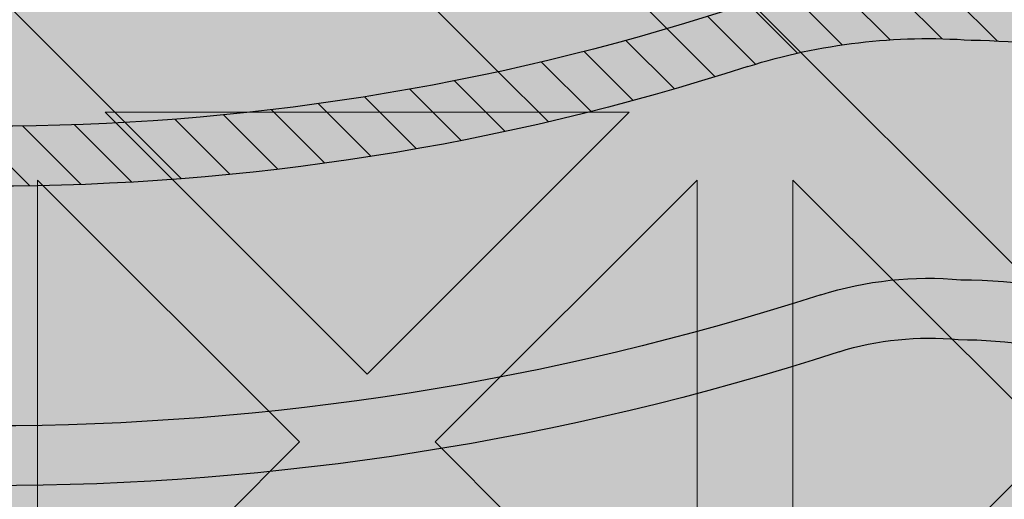
# Model space of a CAD drawing. Units: inches. Extents: x 844 to 2234, y 346 to 1084.
# Tile 28 of 93: x 1257.455 to 1260.074, y 687.38 to 688.657. Entities that reach past the tile are written whole.
import ezdxf

# ---------------------------------------------------------------- set-up
doc = ezdxf.new("R2010")
doc.units = ezdxf.units.IN
doc.header["$MEASUREMENT"] = 0
doc.layers.add('furniture', color=8, linetype='Continuous', lineweight=18)
doc.layers.add('RA-AP-01$0$INT', color=35, linetype='Continuous', lineweight=5)
doc.layers.add('RA-AP-01$0$FURN', color=3, linetype='Continuous')
doc.layers.add('RA-AP-01$0$WOOD', color=64, linetype='Continuous')

# ---------------------------------------------------------------- blocks, each defined once
blk = doc.blocks.new('A$C18D01794')
at = {"layer": 'RA-AP-01$0$INT'}
h = blk.add_hatch(color=256, dxfattribs=at)
h.paths.add_polyline_path([(4.585917135068449, -6.356712009588271), (4.555206456959269, -6.35671200958746), (4.555206456959137, -6.387422687716308), (4.874495778835233, -6.706712009592356), (4.90520645695423, -6.676001331474049)])
h.paths.add_polyline_path([(5.255206456948813, -6.387422687716306), (5.255206456948682, -6.356712009605972), (5.224495778822613, -6.356712009605161), (4.905206456953498, -6.676001331474273), (4.935917135072151, -6.706712009592924)])
h.paths.add_polyline_path([(4.935917135072559, -6.706712009592068), (4.905206456953564, -6.737422687710376), (5.255206456951813, -7.087422687708613), (5.255206456951549, -7.026001331471008)])
h.paths.add_polyline_path([(4.555206456956399, -7.026001331471013), (4.555206456956134, -7.087422687708616), (4.905206456953821, -6.737422687710943), (4.874495778835166, -6.70671200959229)])
h = blk.add_hatch(color=256, dxfattribs=at)
h.paths.add_polyline_path([(4.585917135068448, -6.356712009588273), (4.614201406330596, -6.356712009589021), (4.668846067270487, -6.411356670531338), (4.723490728212344, -6.356712009591912), (4.771774999457151, -6.35671200959319), (4.826419660396886, -6.411356670535356), (4.862780050090322, -6.374996280843536), (4.844495778842715, -6.356712009595112), (4.862780050090411, -6.356712009595595), (4.905206456960182, -6.399138416468211), (4.947632863832445, -6.356712009597838), (4.965917135079675, -6.356712009598322), (4.947632863831759, -6.374996280845421), (4.983993253523576, -6.411356670538857), (5.038637914464627, -6.356712009600247), (5.08692218571208, -6.356712009601523), (5.141566846649976, -6.411356670541852), (5.196211507589851, -6.356712009604411), (5.224495778822615, -6.356712009605161), (4.905206456953975, -6.676001331473793)])
h.paths.add_polyline_path([(4.895206456956031, -6.637717060225675), (4.895206456958921, -6.528427738347902), (4.840561796018589, -6.583072399285802)], flags=16)
h.paths.add_polyline_path([(4.915206456955638, -6.637717060226121), (4.969851117895509, -6.583072399288678), (4.915206456957609, -6.528427738348344)], flags=16)
h.paths.add_polyline_path([(4.826419660395175, -6.568930263661755), (4.881064321335613, -6.514285602723745), (4.771774999456703, -6.514285602720857)], flags=16)
h.paths.add_polyline_path([(4.983993253519558, -6.568930263665262), (5.038637914460456, -6.514285602726792), (4.929348592581548, -6.514285602724816)], flags=16)
h.paths.add_polyline_path([(4.881064321336025, -6.494285602723742), (4.826419660397532, -6.439640941782821), (4.771774999457062, -6.494285602720859)], flags=16)
h.paths.add_polyline_path([(4.929348592582019, -6.494285602724817), (5.038637914460982, -6.494285602726792), (4.983993253522945, -6.439640941786327)], flags=16)
h.paths.add_polyline_path([(4.895206456960191, -6.480143467100443), (4.895206456962115, -6.407422687715913), (4.876922185715016, -6.389138416467584), (4.840561796021581, -6.425498806159401)], flags=16)
h.paths.add_polyline_path([(4.915206456958487, -6.480143467100889), (4.969851117899527, -6.425498806162279), (4.933490728206909, -6.389138416468043), (4.9152064569598, -6.40742268771434)], flags=16)
h.paths.add_polyline_path([(4.757632863832376, -6.480143467096812), (4.812277524772842, -6.425498806158772), (4.757632863834348, -6.370854145217844)], flags=16)
h.paths.add_polyline_path([(4.737632863832376, -6.480143467096286), (4.737632863834348, -6.370854145217375), (4.682988202893906, -6.425498806155385)], flags=16)
h.paths.add_polyline_path([(5.05278005008503, -6.480143467103376), (5.052780050087917, -6.370854145224413), (4.998135389146995, -6.425498806162908)], flags=16)
h.paths.add_polyline_path([(5.072780050085024, -6.480143467103744), (5.127424711025931, -6.42549880616527), (5.072780050087916, -6.370854145224832)], flags=16)
h.paths.add_polyline_path([(4.935917135072783, -6.706712009592292), (5.255206456948811, -6.387422687716309), (5.255206456948932, -6.415706958964177), (5.200561796010279, -6.470351619902839), (5.255206456949403, -6.524996280841948), (5.25520645694961, -6.5732805520894), (5.200561796009787, -6.627925213029239), (5.236922185702417, -6.664285602721864), (5.255206456949919, -6.646001331474357), (5.255206456949998, -6.664285602721898), (5.212780050078687, -6.706712009592262), (5.25520645695036, -6.749138416463932), (5.255206456950438, -6.767422687711313), (5.236922185702424, -6.749138416463297), (5.200561796009796, -6.785498806155928), (5.255206456950753, -6.840143467096874), (5.25520645695096, -6.888427738341682), (5.200561796010322, -6.943072399282328), (5.255206456951428, -6.997717060223427), (5.255206456951547, -7.026001331471006)])
h.paths.add_polyline_path([(5.042988202883395, -6.785498806155427), (5.097632863823085, -6.840143467095101), (5.097632863822622, -6.730854145216193)], flags=16)
h.paths.add_polyline_path([(5.028846067259663, -6.771356670531693), (5.083490728198774, -6.716712009592573), (4.974201406321001, -6.716712009593042)], flags=16)
h.paths.add_polyline_path([(5.117632863823087, -6.840143467095186), (5.172277524762331, -6.785498806155926), (5.11763286382262, -6.730854145216225)], flags=16)
h.paths.add_polyline_path([(5.08349072819877, -6.696712009593886), (5.028846067259652, -6.642067348654775), (4.974201406320998, -6.696712009593438)], flags=16)
h.paths.add_polyline_path([(5.131774999446817, -6.854285602718917), (5.186419660386065, -6.799640941779662), (5.241064321325782, -6.854285602719365)], flags=17)
h.paths.add_polyline_path([(5.131774999446228, -6.716712009592374), (5.186419660386065, -6.771356670532194), (5.222780050079488, -6.734996280838764), (5.204495778832781, -6.716712009592063)], flags=16)
h.paths.add_polyline_path([(5.097632863822613, -6.682569873970264), (5.097632863823061, -6.573280552091354), (5.042988202883383, -6.627925213031044)], flags=16)
h.paths.add_polyline_path([(5.131774999446899, -6.874285602718915), (5.241064321325809, -6.874285602719364), (5.186419660386591, -6.928930263658598)], flags=17)
h.paths.add_polyline_path([(5.131774999446226, -6.696712009594078), (5.204495778830767, -6.696712009594374), (5.22278005007868, -6.67842773834687), (5.186419660386049, -6.642067348654249)], flags=16)
h.paths.add_polyline_path([(5.11763286382262, -6.682569873970225), (5.17227752476232, -6.627925213030515), (5.117632863823064, -6.573280552091267)], flags=16)
h.paths.add_polyline_path([(5.186419660386069, -6.613783077405491), (5.241064321325754, -6.559138416465795), (5.131774999446791, -6.559138416466263)], flags=16)
h.paths.add_polyline_path([(5.131774999446872, -6.539138416466263), (5.24106432132578, -6.539138416465794), (5.186419660386554, -6.484493755526573)], flags=16)
h.paths.add_polyline_path([(5.255206456951811, -7.08742268770861), (5.255206456951895, -7.106712009588038), (4.555206456956052, -7.106712009588038), (4.555206456956136, -7.087422687708617), (4.905206456953973, -6.737422687710788)])
h.paths.add_polyline_path([(4.983993253513404, -6.8444937555241), (4.92934859257295, -6.899138416462108), (5.03863791445186, -6.899138416465014)], flags=16)
h.paths.add_polyline_path([(4.969851117889988, -6.83035161990006), (4.915206456952556, -6.775706958960171), (4.915206456949648, -6.884996280837944)], flags=16)
h.paths.add_polyline_path([(4.929348592572535, -6.919138416462105), (4.983993253511019, -6.973783077403037), (5.038637914451496, -6.919138416465012)], flags=16)
h.paths.add_polyline_path([(5.052780050074912, -6.93328055208906), (4.998135389134438, -6.987925213027088), (5.052780050072919, -7.042569873968025)], flags=16)
h.paths.add_polyline_path([(5.07278005007491, -6.933280552089588), (5.072780050072918, -7.042569873968497), (5.127424711013374, -6.987925213030498)], flags=16)
h.paths.add_polyline_path([(4.89520645695295, -6.775706958959721), (4.840561796013067, -6.830351619897157), (4.895206456950961, -6.884996280837494)], flags=16)
h.paths.add_polyline_path([(4.915206456948365, -6.933280552085403), (4.915206456946434, -7.006001331471951), (4.933490728192729, -7.024285602719066), (4.969851117886972, -6.987925213026453)], flags=16)
h.paths.add_polyline_path([(4.881064321327021, -6.899138416461022), (4.82641966038902, -6.84449375552057), (4.771774999448108, -6.899138416459029)], flags=16)
h.paths.add_polyline_path([(4.895206456950073, -6.933280552084951), (4.840561796009022, -6.987925213023558), (4.876922185700835, -7.024285602716997), (4.895206456948749, -7.006001331469487)], flags=16)
h.paths.add_polyline_path([(4.983993253510392, -7.0020673486505), (4.947632863816944, -7.038427738342319), (4.965917135064043, -7.05671200959023), (5.038637914448995, -7.056712009591555)], flags=16)
h.paths.add_polyline_path([(4.881064321326543, -6.91913841646102), (4.771774999447578, -6.919138416459031), (4.826419660385607, -6.973783077399508)], flags=16)
h.paths.add_polyline_path([(4.905206456946447, -7.014285602717636), (4.862780050074785, -7.056712009588352), (4.947632863816685, -7.056712009589775)], flags=16)
h.paths.add_polyline_path([(5.14156684663679, -7.002067348654549), (5.086922185696452, -7.056712009592438), (5.196211507574223, -7.056712009594425)], flags=16)
h.paths.add_polyline_path([(4.8264196603837, -7.002067348646972), (4.771774999442643, -7.056712009585575), (4.8444957788276, -7.056712009587508), (4.862780050075511, -7.038427738340416)], flags=16)
h.paths.add_polyline_path([(4.812277524760289, -6.98792521302292), (4.757632863822258, -6.933280552082447), (4.757632863819352, -7.042569873961408)], flags=16)
h.paths.add_polyline_path([(4.73763286382226, -6.933280552082079), (4.682988202881349, -6.987925213020536), (4.737632863819352, -7.04256987396099)], flags=16)
h.paths.add_polyline_path([(4.723490728195188, -7.056712009584289), (4.668846067257299, -7.002067348643949), (4.614201406317417, -7.056712009581383)], flags=16)
h.paths.add_polyline_path([(4.597632863829262, -6.706712009592262), (4.555206456957951, -6.664285602721896), (4.555206456958029, -6.646001331474357), (4.573490728205535, -6.664285602721864), (4.609851117898167, -6.627925213029238), (4.555206456958338, -6.573280552089402), (4.555206456958546, -6.524996280841952), (4.60985111789767, -6.470351619902839), (4.555206456959015, -6.415706958964177), (4.555206456959138, -6.387422687716309), (4.874495778835167, -6.70671200959229), (4.5552064569564, -7.026001331471015), (4.555206456956523, -6.997717060223433), (4.609851117897629, -6.94307239928233), (4.555206456956988, -6.888427738341681), (4.555206456957198, -6.840143467096881), (4.609851117898153, -6.78549880615593), (4.573490728205528, -6.749138416463297), (4.555206456957507, -6.76742268771132), (4.555206456957585, -6.749138416463933)])
h.paths.add_polyline_path([(4.712780050085332, -6.730854145216195), (4.712780050084863, -6.840143467095105), (4.767424711024555, -6.785498806155427)], flags=16)
h.paths.add_polyline_path([(4.726922185709173, -6.716712009592573), (4.781566846648288, -6.771356670531693), (4.836211507586949, -6.716712009593043)], flags=16)
h.paths.add_polyline_path([(4.692780050085327, -6.730854145216225), (4.638135389145619, -6.785498806155928), (4.692780050084865, -6.840143467095185)], flags=16)
h.paths.add_polyline_path([(4.726922185709182, -6.696712009593886), (4.836211507586949, -6.696712009593436), (4.7815668466483, -6.642067348654773)], flags=16)
h.paths.add_polyline_path([(4.678637914461726, -6.71671200959237), (4.605917135075169, -6.716712009592063), (4.587632863828464, -6.734996280838766), (4.623993253521887, -6.771356670532195)], flags=16)
h.paths.add_polyline_path([(4.712780050085336, -6.68256987397026), (4.767424711024568, -6.627925213031042), (4.71278005008489, -6.573280552091352)], flags=16)
h.paths.add_polyline_path([(4.678637914461726, -6.696712009594076), (4.623993253521899, -6.642067348654247), (4.587632863829271, -6.67842773834687), (4.605917135077185, -6.696712009594376)], flags=16)
h.paths.add_polyline_path([(4.692780050085336, -6.682569873970228), (4.692780050084889, -6.573280552091267), (4.638135389145632, -6.627925213030515)], flags=16)
h.paths.add_polyline_path([(4.623993253521885, -6.799640941779662), (4.678637914461131, -6.854285602718915), (4.56934859258217, -6.854285602719365)], flags=17)
h.paths.add_polyline_path([(4.623993253521901, -6.613783077405509), (4.678637914461158, -6.559138416466263), (4.569348592582195, -6.559138416465795)], flags=16)
h.paths.add_polyline_path([(4.678637914461051, -6.874285602718915), (4.623993253521361, -6.928930263658598), (4.569348592582143, -6.874285602719364)], flags=17)
h.paths.add_polyline_path([(4.678637914461076, -6.539138416466263), (4.623993253521399, -6.484493755526573), (4.569348592582167, -6.539138416465796)], flags=16)
h = blk.add_hatch(color=256, dxfattribs=at)
h.paths.add_polyline_path([(4.969851117891331, -6.583072399286455), (4.915206456952669, -6.63771706022511), (4.915206456952222, -6.528427738347337)])
h.paths.add_polyline_path([(4.895206456953064, -6.637717060225108), (4.840561796014413, -6.583072399286448), (4.895206456953533, -6.528427738347335)])
h.paths.add_polyline_path([(4.826419660390684, -6.568930263662714), (4.771774999451003, -6.514285602723024), (4.881064321329913, -6.514285602723489)])
h.paths.add_polyline_path([(4.881064321329884, -6.494285602723492), (4.771774999450921, -6.494285602723024), (4.82641966039018, -6.439640941783778)])
h.paths.add_polyline_path([(4.895206456953734, -6.48014346709988), (4.840561796013912, -6.425498806160046), (4.876922185707337, -6.389138416466622), (4.895206456954043, -6.40742268771333)])
h.paths.add_polyline_path([(4.862780050082808, -6.374996280843689), (4.826419660390178, -6.411356670536314), (4.771774999450351, -6.356712009596481), (4.844495778835303, -6.356712009596181)])
h.paths.add_polyline_path([(4.812277524766446, -6.425498806160041), (4.757632863827191, -6.480143467099289), (4.757632863826741, -6.370854145220329)])
h.paths.add_polyline_path([(4.737632863827191, -6.480143467099214), (4.682988202887508, -6.425498806159518), (4.737632863826743, -6.370854145220299)])
h.paths.add_polyline_path([(4.668846067263777, -6.41135667053579), (4.614201406325123, -6.356712009597128), (4.723490728202894, -6.356712009596675)])
h.paths.add_polyline_path([(4.905206456953846, -6.399138416467422), (4.862780050082654, -6.356712009596229), (4.947632863824561, -6.356712009595756)])
h.paths.add_polyline_path([(4.915206456952028, -6.480143467099882), (4.91520645695173, -6.407422687715346), (4.933490728199234, -6.389138416467428), (4.96985111789186, -6.425498806160055)])
h.paths.add_polyline_path([(5.038637914454841, -6.494285602723048), (4.929348592575874, -6.494285602723497), (4.983993253515593, -6.439640941783787)])
h.paths.add_polyline_path([(4.983993253515065, -6.568930263662725), (4.929348592575849, -6.514285602723495), (5.038637914454755, -6.514285602723045)])
h.paths.add_polyline_path([(5.052780050079843, -6.480143467099317), (4.998135389140595, -6.425498806160058), (5.052780050080309, -6.370854145220356)])
h.paths.add_polyline_path([(4.983993253516868, -6.411356670536324), (4.947632863824241, -6.374996280843694), (4.965917135071747, -6.356712009596188), (5.038637914456701, -6.356712009596504)])
h.paths.add_polyline_path([(5.127424711019533, -6.425498806159557), (5.072780050079843, -6.480143467099239), (5.07278005008031, -6.370854145220326)])
h.paths.add_polyline_path([(5.141566846643269, -6.411356670535829), (5.086922185704154, -6.356712009596707), (5.196211507581929, -6.356712009597176)])
for p, q in [((4.905206456953975, -6.676001331473793), (4.585917135071132, -6.356712009590955)), ((4.737632863834348, -6.370854145217375), (4.682988202893906, -6.425498806155385)), ((4.737632863832376, -6.480143467096285), (4.737632863834348, -6.370854145217375)), ((4.757632863832376, -6.48014346709681), (4.757632863834348, -6.370854145217847)), ((4.757632863834348, -6.370854145217847), (4.812277524772842, -6.425498806158774)), ((4.840561796021581, -6.425498806159403), (4.876922185715016, -6.389138416467584)), ((4.895206456962113, -6.407422687715495), (4.895206456960191, -6.480143467100447)), ((4.682988202893908, -6.425498806155387), (4.737632863832376, -6.480143467096285)), ((4.757632863832376, -6.48014346709681), (4.812277524772842, -6.425498806158774)), ((4.895206456960191, -6.480143467100447), (4.840561796021581, -6.425498806159401)), ((4.771774999457064, -6.494285602720857), (4.826419660397532, -6.439640941782821)), ((4.881064321336027, -6.494285602723744), (4.826419660397532, -6.439640941782821)), ((4.771774999457064, -6.494285602720857), (4.881064321336027, -6.494285602723744))]:
    blk.add_line(p, q, dxfattribs=at)
blk = doc.blocks.new('A$C32926AE1')
at = {"layer": 'RA-AP-01$0$WOOD'}
h = blk.add_hatch(color=256, dxfattribs=at)
h.dxf.hatch_style = 1
h.paths.add_polyline_path([(5.157430609644524, 4.573483066760929, -0.1009492694046607), (5.155401577623758, 4.593365984175333, -0.1842662638101597), (5.172249623284174, 4.638795604568598, 0.2056608120311276), (5.179560981299304, 4.661316324430096, 0.3614336704623542), (5.134352340494423, 4.706524965234944, 0.2056608120311297), (5.111831620632933, 4.699213607219793, -0.1842662638101113), (5.066402000239693, 4.682365561559342, -0.1055311479399994), (5.045656153913092, 4.68467289944697, 0.1567636581983829), (4.763886414745334, 4.684672899446966, -0.1055311479399895), (4.743140568418733, 4.68236556155934, -0.1842662638100833), (4.6977109480255, 4.69921360721979, 0.2056608120302612), (4.675190228164109, 4.706524965234949, 0.3614336704708441), (4.629981587358889, 4.66131632442871, 0.2056608120245944), (4.637292945374126, 4.638795604567974, -0.1842662638101024), (4.654140991034615, 4.59336598417475, -0.1009492694055169), (4.652111959013835, 4.573483066760181, 0.021410119221476), (4.629748025606143, 4.156712009541676, 0.0214101192214795), (4.652111959013809, 3.739940952323101, -0.1009492694059586), (4.654140991034615, 3.720058034908448, -0.1842662638100975), (4.637292945374126, 3.674628414515226, 0.2056608120245705), (4.629981587358889, 3.652107694654492, 0.3614336704708879), (4.675190228164113, 3.606899053848249, 0.2056608120302384), (4.697710948025501, 3.614210411863408, -0.1842662638100995), (4.743140568418738, 3.63105845752386, -0.1055311479402541), (4.763886414745388, 3.628751119636215, 0.1567636581983776), (5.045656153913137, 3.628751119636244, -0.1055311479397538), (5.066402000239692, 3.631058457523857, -0.1842662638101067), (5.111831620632931, 3.614210411863407, 0.2056608120310924), (5.134352340494417, 3.606899053848256, 0.3614336704624001), (5.179560981299307, 3.652107694653103, 0.2056608120311314), (5.172249623284175, 3.6746284145146, -0.1842662638101402), (5.155401577623758, 3.72005803490786, -0.1009492694051366), (5.15743060964455, 3.739940952322354, 0.0214101192215073), (5.179794543052287, 4.156712009541468, 0.0214101192215252)])
h.paths.add_polyline_path([(4.639748609479751, 4.156712009541513, 0.0213537860821624), (4.661970494867118, 3.741887061152232, -0.094075836301374), (4.664143710413708, 3.7196126951003, -0.1824818158568985), (4.644813765429836, 3.668037719127816, 0.2056608120245319), (4.639939526753007, 3.653023905887301, 0.3614336704710246), (4.676106439397173, 3.616856993242342, 0.2056608120302234), (4.691120252638095, 3.621731231919122, -0.1824818158602558), (4.742695228611606, 3.641061176902986, -0.1029891339458722), (4.766991894714349, 3.638256818950944, 0.156709409989566), (5.042550673941472, 3.638256818950105, -0.102989133958497), (5.066847340047078, 3.641061176902949, -0.1824818158594995), (5.118422316020358, 3.621731231919103, 0.2056608120311416), (5.133436129261316, 3.616856993242346, 0.3614336704621468), (5.169603041905217, 3.653023905886178, 0.2056608120310986), (5.164728803228477, 3.668037719127177, -0.1824818158565612), (5.145398858244737, 3.719612695099578, -0.0940758363009313), (5.147572073791232, 3.741887061151398, 0.0213537860822023), (5.169793959178681, 4.156712009541451, 0.0213537860822226), (5.147572073791203, 4.571536957931898, -0.0940758363005034), (5.145398858244737, 4.59381132398362, -0.1824818158565587), (5.164728803228476, 4.645386299956021, 0.2056608120311045), (5.169603041905216, 4.66040011319702, 0.3614336704621845), (5.133436129261313, 4.696567025840856, 0.2056608120310773), (5.118422316020359, 4.691692787164098, -0.182481815859508), (5.066847340047078, 4.67236284218025, -0.1029891339584606), (5.04255067394148, 4.675167200133092, 0.156709409989566), (4.766991894714357, 4.675167200132257, -0.1029891339458842), (4.742695228611611, 4.672362842180213, -0.1824818158602725), (4.691120252638095, 4.691692787164077, 0.2056608120302152), (4.676106439397174, 4.696567025840858, 0.3614336704710363), (4.639939526753005, 4.660400113195899, 0.2056608120245495), (4.644813765429837, 4.645386299955384, -0.1824818158568934), (4.664143710413708, 4.593811323982902, -0.0940758363009187), (4.661970494867149, 4.571536957931074, 0.021353786082177)], flags=16)
h.paths.add_polyline_path([(5.129794543052235, 4.432167055276933, -0.0141661062790638), (5.130152669293814, 4.156927903047693, -0.0141661062790647), (5.129794543052234, 3.881688750818433, -0.0785247771143638), (5.10979738006795, 3.755143611847103, 0.0945969212073497), (5.105408519571111, 3.717898134952927, 0.1043170707844957), (5.116074640131521, 3.670385395016088, 0.1043170707864965), (5.068561900193738, 3.681051515576561, 0.09459692119553), (5.031316423304057, 3.676662655080835, -0.1580239521427272), (4.778226145355827, 3.676662655080367, 0.0945969211986668), (4.740980668464973, 3.681051515576592, 0.1043170707882822), (4.693467928526415, 3.670385395015844, 0.1043170707867916), (4.704134049087309, 3.717898134953662, 0.0945969211972894), (4.69974518859162, 3.755143611844042, -0.0785247771163196), (4.679748025606343, 3.881688750818406, -0.0141661062790663), (4.679389899364763, 4.156927903047693, -0.0141661062790672), (4.679748025606343, 4.432167055276998, -0.0785247771163064), (4.699745188591625, 4.55871219425134, 0.094596921197333), (4.704134049087308, 4.595957671141738, 0.1043170707867205), (4.693467928526416, 4.643470411079523, 0.1043170707882628), (4.740980668464965, 4.632804290518776, 0.0945969211988114), (4.778226145355874, 4.637193151015016, -0.158023952142669), (5.031316423304015, 4.637193151014546, 0.0945969211956361), (5.068561900193736, 4.632804290518806, 0.1043170707864979), (5.11607464013152, 4.643470411079278, 0.1043170707844617), (5.105408519571112, 4.595957671142455, 0.0945969212074597), (5.109797380067959, 4.558712194248236, -0.0785247771143467)], flags=0)
h.paths.add_polyline_path([(5.119794532311105, 4.432259799204851, -0.0142000800617244), (5.120156169157484, 4.156927903047701, -0.0142000800617277), (5.119794532311105, 3.881596006890482, -0.0784894509520253), (5.100273383573699, 3.758192358677797, 0.0940138827242913), (5.095413455884425, 3.717477693979438, 0.0606271852308753), (5.099615656341024, 3.686844378806616, 0.0606271852322524), (5.068982341167493, 3.691046579263239, 0.0940138827010453), (5.028267676478798, 3.686186651576848, -0.1580706864508061), (4.781274892180912, 3.686186651576435, 0.0940138827026903), (4.740560227491556, 3.691046579263279, 0.0606271852339895), (4.709926912317155, 3.686844378806508, 0.0606271852329405), (4.714129112773991, 3.717477693980356, 0.094013882701304), (4.709269185087677, 3.758192358669163, -0.0784894509577193), (4.689748036347473, 3.881596006890469, -0.014200080061729), (4.689386399501094, 4.156927903047709, -0.0142000800617217), (4.689748036347473, 4.432259799204808, -0.078489450957724), (4.709269185087651, 4.555663447426125, 0.0940138827014585), (4.714129112773992, 4.596378112114996, 0.0606271852329731), (4.709926912317154, 4.62701142728886, 0.0606271852340196), (4.74056022749157, 4.622809226832087, 0.0940138827024997), (4.781274892180847, 4.627669154518912, -0.1580706864508359), (5.028267676478777, 4.627669154518526, 0.0940138827010946), (5.068982341167492, 4.622809226832129, 0.060627185232254), (5.099615656341024, 4.627011427288751, 0.0606271852308727), (5.095413455884425, 4.59637811211593, 0.0940138827241088), (5.100273383573675, 4.555663447417647, -0.0784894509520978)], flags=0)
h.paths.add_polyline_path([(5.06978912287499, 4.430218106756144, -0.014241683694547), (5.070173729147532, 4.156927903047672, -0.0142416836945458), (5.06978912287499, 3.883637699339223, -0.0800609523125196), (5.052662118612511, 3.773463122773442, 0.0526421978001116), (5.04590916754064, 3.740550867606997, 0.0526421977992423), (5.012996912374707, 3.73379791653534, -0.1583028414718258), (4.796545656286308, 3.73379791653451, 0.0526421978034211), (4.763633401117837, 3.740550867607021, 0.0526421978018622), (4.756880450045755, 3.773463122774558, -0.0800609523117106), (4.739753445783639, 3.883637699339268, -0.0142416836945435), (4.739368839511098, 4.156927903047671, -0.0142416836945477), (4.739753445783639, 4.430218106756155, -0.0800609523116345), (4.75688045004574, 4.540392683320762, 0.052642197801941), (4.763633401117837, 4.573304938488346, 0.0526421978035071), (4.796545656286361, 4.580057889560873, -0.1583028414717561), (5.012996912374669, 4.580057889560039, 0.0526421977993048), (5.04590916754064, 4.57330493848837, 0.0526421978002057), (5.052662118612529, 4.540392683321868, -0.080060952312477)], flags=0)
h.paths.add_polyline_path([(5.049789715110557, 4.43038092723357, -0.0143097550741839), (5.05018085590259, 4.156927903047715, -0.0143097550741854), (5.049789715110558, 3.883474878861827, -0.0800685599149176), (5.03362098255317, 3.779581877367999, 0.0306258898956367), (5.028241146483733, 3.758218888663947, 0.0306258898977031), (5.006878157778253, 3.75283905259408, -0.1583983521624096), (4.802664410878162, 3.752839052594731, 0.0306258898946014), (4.781301422174808, 3.758218888663924, 0.0306258898967912), (4.775921586105202, 3.779581877368794, -0.080068559914251), (4.759752853548071, 3.883474878861786, -0.0143097550741854), (4.759361712756037, 4.156927903047671, -0.0143097550741854), (4.759752853548071, 4.430380927233557, -0.0800685599142479), (4.775921586105193, 4.534273928726546, 0.0306258898968306), (4.781301422174808, 4.555636917431444, 0.0306258898945754), (4.802664410878143, 4.561016753500631, -0.1583983521624168), (5.006878157778244, 4.561016753501291, 0.0306258898977177), (5.028241146483733, 4.555636917431421, 0.0306258898958182), (5.03362098255321, 4.534273928727244, -0.080068559914796)], flags=0)
h.paths.add_polyline_path([(4.999766070382627, 4.428171244713864, -0.0143443147609634), (5.000198441819402, 4.156927903047689, -0.0143443147609612), (4.999766070382627, 3.885684561381556, -0.0784641635803329), (4.987356730658798, 3.799103304488872, -0.1506053783831347), (4.822185837999821, 3.79910330448882, -0.0784641635803318), (4.809776498276007, 3.885684561381509, -0.014344314760963), (4.809344126839227, 4.156927903047677, -0.0143443147609645), (4.809776498276007, 4.428171244713873, -0.0784641635803192), (4.822185837999822, 4.514752501606549, -0.1506053783831338), (4.987356730658798, 4.514752501606494, -0.078464163580285)], flags=0)
h.paths.add_polyline_path([(4.979755254238824, 4.42764379880488, -0.0143772539198268), (4.980205517789977, 4.156927903047693, -0.0143772539198275), (4.979755254238824, 3.886212007290489, -0.0689242507424422), (4.971183264704897, 3.815276770442801, -0.1296645318904179), (4.838359303953726, 3.815276770442746, -0.0689242507424186), (4.829787314419809, 3.886212007290419, -0.0143772539198292), (4.829337050868653, 4.156927903047653, -0.0143772539198325), (4.829787314419809, 4.427643798804946, -0.0689242507424211), (4.838359303953725, 4.498579035652621, -0.1296645318904187), (4.971183264704897, 4.498579035652565, -0.0689242507424401)], flags=0)
h = blk.add_hatch(color=256, dxfattribs=at)
h.dxf.hatch_style = 1
h.paths.add_polyline_path([(5.145398858244737, 4.59381132398362, -0.1824818158565616), (5.164728803228476, 4.645386299956021, 0.2056608120311045), (5.169603041905216, 4.66040011319702, 0.3614336704621845), (5.133436129261313, 4.696567025840856, 0.2056608120310773), (5.118422316020359, 4.691692787164098, -0.182481815859508), (5.066847340047078, 4.67236284218025, -0.1029891339584606), (5.04255067394148, 4.675167200133092, 0.156709409989566), (4.766991894714357, 4.675167200132257, -0.1029891339458842), (4.742695228611611, 4.672362842180213, -0.1824818158602725), (4.691120252638095, 4.691692787164077, 0.2056608120302152), (4.676106439397174, 4.696567025840858, 0.3614336704710363), (4.639939526753005, 4.660400113195899, 0.2056608120245495), (4.644813765429837, 4.645386299955384, -0.1824818158568934), (4.664143710413708, 4.593811323982902, -0.0940758363009187), (4.661970494867149, 4.571536957931074, 0.0213537860821772), (4.639748609479751, 4.156712009541507, 0.0213537860821625), (4.661970494867119, 3.741887061152226, -0.0940758363013071), (4.664143710413708, 3.719612695100309, -0.1824818158569294), (4.644813765429836, 3.668037719127816, 0.2056608120245319), (4.639939526753007, 3.653023905887301, 0.3614336704710246), (4.676106439397173, 3.616856993242342, 0.2056608120302234), (4.691120252638095, 3.621731231919122, -0.1824818158602558), (4.742695228611606, 3.641061176902986, -0.1029891339458722), (4.766991894714349, 3.638256818950944, 0.156709409989566), (5.042550673941472, 3.638256818950105, -0.102989133958497), (5.066847340047078, 3.641061176902949, -0.1824818158594995), (5.118422316020358, 3.621731231919103, 0.2056608120311416), (5.133436129261316, 3.616856993242346, 0.3614336704621468), (5.169603041905217, 3.653023905886178, 0.2056608120310986), (5.164728803228477, 3.668037719127177, -0.1824818158565612), (5.145398858244737, 3.719612695099578, -0.0940758363009313), (5.147572073791232, 3.741887061151398, 0.0213537860822023), (5.169793959178681, 4.156712009541451, 0.0213537860822226), (5.147572073791203, 4.571536957931898, -0.0940758363004996)])
h.paths.add_polyline_path([(5.109797380067958, 4.55871219424824, -0.0785247771143472), (5.129794543052234, 4.432167055276936, -0.0141661062790644), (5.130152669293814, 4.156927903047685, -0.014166106279066), (5.129794543052234, 3.881688750818401, -0.0785247771143517), (5.109797380067946, 3.755143611847092, 0.0945969212073132), (5.105408519571111, 3.717898134952929, 0.1043170707844995), (5.116074640131521, 3.670385395016088, 0.1043170707864965), (5.068561900193738, 3.681051515576561, 0.09459692119553), (5.031316423304057, 3.676662655080835, -0.1580239521427272), (4.778226145355827, 3.676662655080367, 0.0945969211986668), (4.740980668464973, 3.681051515576592, 0.1043170707882822), (4.693467928526415, 3.670385395015844, 0.1043170707867916), (4.704134049087309, 3.717898134953662, 0.0945969211972894), (4.69974518859162, 3.755143611844042, -0.0785247771163196), (4.679748025606343, 3.881688750818406, -0.0141661062790663), (4.679389899364763, 4.156927903047693, -0.0141661062790672), (4.679748025606343, 4.432167055276998, -0.0785247771163064), (4.699745188591625, 4.55871219425134, 0.094596921197333), (4.704134049087308, 4.595957671141738, 0.1043170707867205), (4.693467928526416, 4.643470411079523, 0.1043170707882628), (4.740980668464965, 4.632804290518776, 0.0945969211988114), (4.778226145355874, 4.637193151015016, -0.158023952142669), (5.031316423304015, 4.637193151014546, 0.0945969211956361), (5.068561900193736, 4.632804290518806, 0.1043170707864979), (5.11607464013152, 4.643470411079278, 0.1043170707844617), (5.105408519571112, 4.595957671142455, 0.0945969212074504)], flags=16)
h.paths.add_polyline_path([(5.100273383573655, 4.55566344741771, -0.0784894509521388), (5.119794532311105, 4.432259799204852, -0.0142000800617252), (5.120156169157484, 4.156927903047686, -0.014200080061726), (5.119794532311105, 3.881596006890502, -0.0784894509520446), (5.100273383573696, 3.758192358677786, 0.0940138827242721), (5.095413455884425, 3.717477693979436, 0.0606271852308692), (5.099615656341024, 3.686844378806616, 0.0606271852322522), (5.068982341167493, 3.691046579263239, 0.0940138827010453), (5.028267676478798, 3.686186651576848, -0.1580706864508061), (4.781274892180912, 3.686186651576435, 0.0940138827026903), (4.740560227491556, 3.691046579263279, 0.0606271852339895), (4.709926912317155, 3.686844378806508, 0.0606271852329405), (4.714129112773991, 3.717477693980356, 0.094013882701304), (4.709269185087677, 3.758192358669163, -0.0784894509577193), (4.689748036347473, 3.881596006890469, -0.014200080061729), (4.689386399501094, 4.156927903047709, -0.0142000800617217), (4.689748036347473, 4.432259799204808, -0.078489450957724), (4.709269185087651, 4.555663447426125, 0.0940138827014585), (4.714129112773992, 4.596378112114996, 0.0606271852329731), (4.709926912317154, 4.62701142728886, 0.0606271852340196), (4.74056022749157, 4.622809226832087, 0.0940138827024997), (4.781274892180847, 4.627669154518912, -0.1580706864508359), (5.028267676478777, 4.627669154518526, 0.0940138827010946), (5.068982341167492, 4.622809226832129, 0.060627185232254), (5.099615656341024, 4.627011427288751, 0.0606271852308727), (5.095413455884425, 4.59637811211593, 0.094013882723957)], flags=0)
h.paths.add_polyline_path([(5.04590916754064, 4.57330493848837, 0.0526421978002057), (5.052662118612529, 4.540392683321868, -0.0800609523124783), (5.06978912287499, 4.430218106756142, -0.0142416836945469), (5.070173729147532, 4.156927903047672, -0.0142416836945458), (5.06978912287499, 3.883637699339223, -0.0800609523125196), (5.052662118612511, 3.773463122773442, 0.0526421978001116), (5.04590916754064, 3.740550867606997, 0.0526421977992423), (5.012996912374707, 3.73379791653534, -0.1583028414718258), (4.796545656286308, 3.73379791653451, 0.0526421978034211), (4.763633401117837, 3.740550867607021, 0.0526421978018622), (4.756880450045755, 3.773463122774558, -0.0800609523117106), (4.739753445783639, 3.883637699339268, -0.0142416836945435), (4.739368839511098, 4.156927903047671, -0.0142416836945477), (4.739753445783639, 4.430218106756155, -0.0800609523116345), (4.75688045004574, 4.540392683320762, 0.052642197801941), (4.763633401117837, 4.573304938488346, 0.0526421978035071), (4.796545656286361, 4.580057889560873, -0.1583028414717561), (5.012996912374669, 4.580057889560039, 0.0526421977993048)], flags=0)
h.paths.add_polyline_path([(5.028241146483733, 4.555636917431422, 0.0306258898956949), (5.033620982553182, 4.534273928727329, -0.0800685599148649), (5.049789715110557, 4.430380927233569, -0.0143097550741839), (5.05018085590259, 4.156927903047715, -0.0143097550741854), (5.049789715110558, 3.883474878861827, -0.0800685599149176), (5.03362098255317, 3.779581877367999, 0.0306258898956367), (5.028241146483733, 3.758218888663947, 0.0306258898977031), (5.006878157778253, 3.75283905259408, -0.1583983521624096), (4.802664410878162, 3.752839052594731, 0.0306258898946014), (4.781301422174808, 3.758218888663924, 0.0306258898967912), (4.775921586105202, 3.779581877368794, -0.080068559914251), (4.759752853548071, 3.883474878861786, -0.0143097550741854), (4.759361712756037, 4.156927903047671, -0.0143097550741854), (4.759752853548071, 4.430380927233557, -0.0800685599142479), (4.775921586105193, 4.534273928726546, 0.0306258898968306), (4.781301422174808, 4.555636917431444, 0.0306258898945754), (4.802664410878143, 4.561016753500631, -0.1583983521624168), (5.006878157778244, 4.561016753501291, 0.0306258898977174)], flags=0)
h.paths.add_polyline_path([(4.987356730658798, 4.514752501606494, -0.0784641635803018), (4.999766070382627, 4.428171244713845, -0.0143443147609637), (5.000198441819402, 4.156927903047665, -0.0143443147609622), (4.999766070382628, 3.885684561381514, -0.0784641635802952), (4.987356730658797, 3.799103304488872, -0.1506053783831338), (4.822185837999821, 3.799103304488819, -0.0784641635803342), (4.809776498276007, 3.885684561381512, -0.0143443147609628), (4.809344126839227, 4.156927903047676, -0.0143443147609646), (4.809776498276007, 4.428171244713873, -0.0784641635803192), (4.822185837999822, 4.514752501606549, -0.1506053783831338)], flags=0)
h.paths.add_polyline_path([(4.971183264704897, 4.498579035652566, -0.0689242507424384), (4.979755254238824, 4.427643798804883, -0.0143772539198276), (4.980205517789977, 4.15692790304768, -0.0143772539198258), (4.979755254238823, 3.88621200729051, -0.0689242507424628), (4.971183264704897, 3.815276770442801, -0.129664531890417), (4.838359303953726, 3.815276770442746, -0.0689242507424186), (4.829787314419809, 3.886212007290419, -0.0143772539198292), (4.829337050868653, 4.156927903047653, -0.0143772539198325), (4.829787314419809, 4.427643798804946, -0.0689242507424211), (4.838359303953725, 4.498579035652621, -0.1296645318904187)], flags=0)
h = blk.add_hatch(dxfattribs=at)
h.set_pattern_fill('ANSI31', color=256, scale=0.05, style=0)
h.set_pattern_definition([(45, (0, 0), (-0.0044194173824159, 0.0044194173824159), [])])
h.paths.add_polyline_path([(5.130152669293814, 4.156927903047704, 0.0141661062790657), (5.129794543052234, 4.432167055276982, 0.0777827904001433), (5.110168979996553, 4.557559993161921, -0.0976515123401879), (5.105408519571111, 4.595957671142454, -0.1043170707844687), (5.116074640131522, 4.64347041107928), (5.099615656341024, 4.627011427288751, 0.0606271852308727), (5.095413455884425, 4.59637811211593, 0.0940138827241088), (5.100273383573675, 4.555663447417647, -0.0784894509520972), (5.119794532311105, 4.432259799204852, -0.0142000800617252), (5.120156169157484, 4.156927903047686, -0.014200080061726), (5.119794532311105, 3.881596006890502, -0.0784894509520446), (5.100273383573696, 3.758192358677786, 0.0940138827242721), (5.095413455884425, 3.717477693979436, 0.0606271852308692), (5.099615656341024, 3.686844378806616), (5.116074640131519, 3.67038539501609, -0.1043170707844594), (5.105408519571112, 3.717898134952912, -0.0976515123401594), (5.11016897999655, 3.756295812933435, 0.0777827904001654), (5.129794543052234, 3.881688750818409, 0.0141661062790665)])
h.paths.add_polyline_path([(5.030164222210597, 3.676291055149937, -0.0976515123472002), (5.068561900193739, 3.681051515576561, -0.1043170707864927), (5.116074640131521, 3.670385395016088), (5.099615656341024, 3.686844378806616, 0.0606271852322522), (5.068982341167493, 3.691046579263239, 0.0940138827010453), (5.028267676478798, 3.686186651576848, -0.1580706864508061), (4.781274892180912, 3.686186651576435, 0.0940138827026903), (4.740560227491556, 3.691046579263279, 0.0606271852339913), (4.709926912317154, 3.686844378806508), (4.693467928526416, 3.670385395015845, -0.1043170707882796), (4.740980668464973, 3.681051515576592, -0.0976515123427246), (4.779378346446416, 3.676291055150394, 0.156512506893803)])
h.paths.add_polyline_path([(4.689748036347473, 3.881596006890472, -0.014200080061729), (4.689386399501094, 4.156927903047712, -0.0142000800617195), (4.689748036347473, 4.432259799204768, -0.078489450957742), (4.709269185087648, 4.555663447426114, 0.0940138827014821), (4.714129112773992, 4.596378112114995, 0.0606271852329748), (4.709926912317154, 4.62701142728886), (4.693467928526414, 4.643470411079524, -0.1043170707867939), (4.704134049087309, 4.595957671141706, -0.09765151234893), (4.699373588660725, 4.557559993157876, 0.0777827903975372), (4.679748025606343, 4.432167055276987, 0.0141661062790675), (4.679389899364763, 4.156927903047675, 0.0141661062790641), (4.679748025606343, 3.88168875081843, 0.0777827903975637), (4.699373588660724, 3.756295812937497, -0.0976515123490278), (4.704134049087308, 3.717898134953629, -0.1043170707867196), (4.693467928526416, 3.670385395015845), (4.709926912317155, 3.686844378806508, 0.0606271852329413), (4.714129112773991, 3.717477693980357, 0.0940138827013084), (4.709269185087676, 3.758192358669166, -0.0784894509577192)])
h.paths.add_polyline_path([(4.779378346446434, 4.63756475094498, -0.0976515123427943), (4.740980668464964, 4.632804290518776, -0.1043170707882609), (4.693467928526416, 4.643470411079523), (4.709926912317154, 4.62701142728886, 0.0606271852340196), (4.74056022749157, 4.622809226832087, 0.0940138827024997), (4.781274892180847, 4.627669154518912, -0.1580706864508359), (5.028267676478777, 4.627669154518526, 0.0940138827010946), (5.068982341167492, 4.622809226832129, 0.060627185232254), (5.099615656341024, 4.627011427288751), (5.116074640131521, 4.643470411079279, -0.1043170707865022), (5.068561900193735, 4.632804290518806, -0.0976515123475899), (5.030164222210446, 4.637564750945479, 0.1565125068936924)])
h = blk.add_hatch(dxfattribs=at)
h.set_pattern_fill('ANSI32', color=256, scale=0.2, style=0)
h.set_pattern_definition([(45, (0, 0), (-0.0530330085889911, 0.0530330085889911), []), (45, (0.035355339, 0), (-0.0530330085889911, 0.0530330085889911), [])])
h.paths.add_polyline_path([(5.119794532311105, 4.432259799204823, 0.0777015974868765), (5.10065834347252, 4.554469821747928, -0.0968902511992216), (5.095413455884425, 4.596378112115931, -0.060627185230871), (5.099615656341024, 4.627011427288751, -0.060627185232254), (5.068982341167492, 4.622809226832129, -0.0968902512198245), (5.027074050790956, 4.628054114423209, 0.1564657949319105), (4.782468517866163, 4.628054114422785, -0.0968902512152247), (4.740560227491555, 4.622809226832088, -0.0606271852339878), (4.709926912317155, 4.627011427288859, -0.0606271852329413), (4.714129112773991, 4.596378112115011, -0.0968902512205338), (4.708884225182929, 4.554469821738175, 0.0777015974804443), (4.689748036347473, 4.43225979920482, 0.0142000800617215), (4.689386399501094, 4.156927903047726, 0.0142000800617273), (4.689748036347473, 3.88159600689052, 0.077701597480541), (4.708884225182985, 3.759385984357019, -0.096890251220082), (4.714129112773992, 3.717477693980371, -0.0606271852329731), (4.709926912317154, 3.686844378806507, -0.060627185233988), (4.740560227491554, 3.691046579263279, -0.0968902512152569), (4.782468517866175, 3.685801691672578, 0.1564657949319236), (5.027074050790988, 3.685801691672169, -0.0968902512197451), (5.068982341167491, 3.691046579263239, -0.0606271852322557), (5.099615656341024, 3.686844378806616, -0.0606271852308727), (5.095413455884425, 3.717477693979438, -0.0968902511991229), (5.100658343472507, 3.7593859843474, 0.0777015974868745), (5.119794532311105, 3.8815960068905, 0.014200080061726), (5.120156169157484, 4.156927903047685, 0.0142000800617238)])
h.paths.add_polyline_path([(5.070173729147531, 4.156927903047684, -0.0142416836945481), (5.06978912287499, 3.883637699339191, -0.0800609523125107), (5.052662118612505, 3.773463122773424, 0.0526421978000811), (5.04590916754064, 3.740550867606997, 0.0526421977993214), (5.012996912374658, 3.733797916535325, -0.1583028414717916), (4.796545656286304, 3.733797916534512, 0.0526421978034138), (4.763633401117837, 3.740550867607021, 0.0526421978018622), (4.756880450045755, 3.773463122774558, -0.0800609523117106), (4.739753445783639, 3.883637699339268, -0.0142416836945435), (4.739368839511098, 4.156927903047671, -0.0142416836945477), (4.739753445783639, 4.430218106756155, -0.0800609523116345), (4.75688045004574, 4.540392683320762, 0.052642197801941), (4.763633401117837, 4.573304938488346, 0.0526421978035071), (4.796545656286361, 4.580057889560873, -0.1583028414717561), (5.012996912374669, 4.580057889560039, 0.0526421977993048), (5.04590916754064, 4.57330493848837, 0.0526421978002057), (5.052662118612529, 4.540392683321868, -0.0800609523124783), (5.06978912287499, 4.430218106756142, -0.0142416836945463)], flags=16)
h.paths.add_polyline_path([(5.050180855902591, 4.156927903047686, -0.0143097550741856), (5.049789715110558, 3.883474878861795, -0.0800685599148126), (5.033620982553202, 3.7795818773681, 0.0306258898957837), (5.028241146483733, 3.758218888663947, 0.0306258898977031), (5.006878157778253, 3.75283905259408, -0.1583983521624096), (4.802664410878162, 3.752839052594731, 0.0306258898946014), (4.781301422174808, 3.758218888663924, 0.0306258898967912), (4.775921586105202, 3.779581877368794, -0.080068559914251), (4.759752853548071, 3.883474878861786, -0.0143097550741854), (4.759361712756037, 4.156927903047671, -0.0143097550741854), (4.759752853548071, 4.430380927233557, -0.0800685599142479), (4.775921586105193, 4.534273928726546, 0.0306258898968306), (4.781301422174808, 4.555636917431444, 0.0306258898945754), (4.802664410878143, 4.561016753500631, -0.1583983521624168), (5.006878157778244, 4.561016753501291, 0.0306258898977177), (5.028241146483733, 4.555636917431421, 0.0306258898958182), (5.03362098255321, 4.534273928727244, -0.0800685599147973), (5.049789715110557, 4.430380927233568, -0.0143097550741854)], flags=0)
h.paths.add_polyline_path([(5.000198441819402, 4.15692790304769, -0.0143443147609622), (4.999766070382627, 3.885684561381539, -0.0784641635803169), (4.987356730658798, 3.799103304488873, -0.1506053783831347), (4.822185837999821, 3.79910330448882, -0.0784641635803318), (4.809776498276007, 3.885684561381509, -0.014344314760963), (4.809344126839227, 4.156927903047677, -0.0143443147609645), (4.809776498276007, 4.428171244713873, -0.0784641635803192), (4.822185837999822, 4.514752501606549, -0.1506053783831338), (4.987356730658798, 4.514752501606494, -0.0784641635803018), (4.999766070382627, 4.428171244713845, -0.0143443147609624)], flags=0)
h.paths.add_polyline_path([(4.980205517789976, 4.156927903047707, -0.0143772539198295), (4.979755254238824, 3.886212007290466, -0.06892425074242), (4.971183264704897, 3.815276770442801, -0.129664531890417), (4.838359303953726, 3.815276770442746, -0.0689242507424186), (4.829787314419809, 3.886212007290419, -0.0143772539198292), (4.829337050868653, 4.156927903047653, -0.0143772539198325), (4.829787314419809, 4.427643798804946, -0.0689242507424211), (4.838359303953725, 4.498579035652621, -0.1296645318904187), (4.971183264704897, 4.498579035652565, -0.0689242507424418), (4.979755254238824, 4.427643798804878, -0.0143772539198259)], flags=0)
for centre, radius, start, end in [((4.904771284329219, 4.067062675376634), 0.4003971832811741, 252.0350753990311, 287.9649246011635), ((4.742507915094493, 3.563091385939261), 0.1179700159630538, 90.74177518688705, 114.563326950074), ((4.748108354051326, 3.581305858537386), 0.1000000000000038, 72.4716349533902, 94.08732888364744), ((4.904771284329219, 4.067062675376636), 0.4103971832811756, 252.0403002450644, 287.9596997551364), ((4.742507915094546, 3.56309138593928), 0.0779700159630463, 89.86235369886275, 131.2289490796796), ((4.748108354051293, 3.581305858537387), 0.0599999999999989, 72.59387295230013, 95.17619216014101), ((4.904771284329217, 4.067062675376635), 0.4503971832811742, 252.0623235132636, 287.9376764870612), ((4.742507915094499, 3.563091385939265), 0.0679700159630274, 89.46669294863285, 131.2289490796463), ((4.748108354051358, 3.58130585853739), 0.0500000000000024, 72.64431602474727, 95.70207076536123), ((4.904771284329219, 4.067062675376637), 0.4603971832811766, 252.0683908477148, 287.9316091522846)]:
    blk.add_arc(centre, radius, start, end, dxfattribs=at)
blk = doc.blocks.new('A$C5D2F253E')
at = {"layer": 'RA-AP-01$0$FURN', "xscale": -0.7999999999883585, "yscale": 0.7999999999883585, "zscale": 0.8, "rotation": 90}
blk.add_blockref('A$C18D01794', (-5.687757199772477, 4.75791982714071), dxfattribs=at)
at = {"layer": 'RA-AP-01$0$WOOD', "rotation": 270}
blk.add_blockref('A$C32926AE1', (-4.161339601644158, 5.73852594588169), dxfattribs=at)

msp = doc.modelspace()

# ---------------------------------------------------------------- block references
at = {"layer": 'furniture', "xscale": -15.94108302203742, "yscale": 15.94108302203742, "zscale": 15.94108302203742, "rotation": 270}
msp.add_blockref('A$C5D2F253E', (1244.08405109492, 696.2584716700112), dxfattribs=at)

doc.saveas('drawing.dxf')
